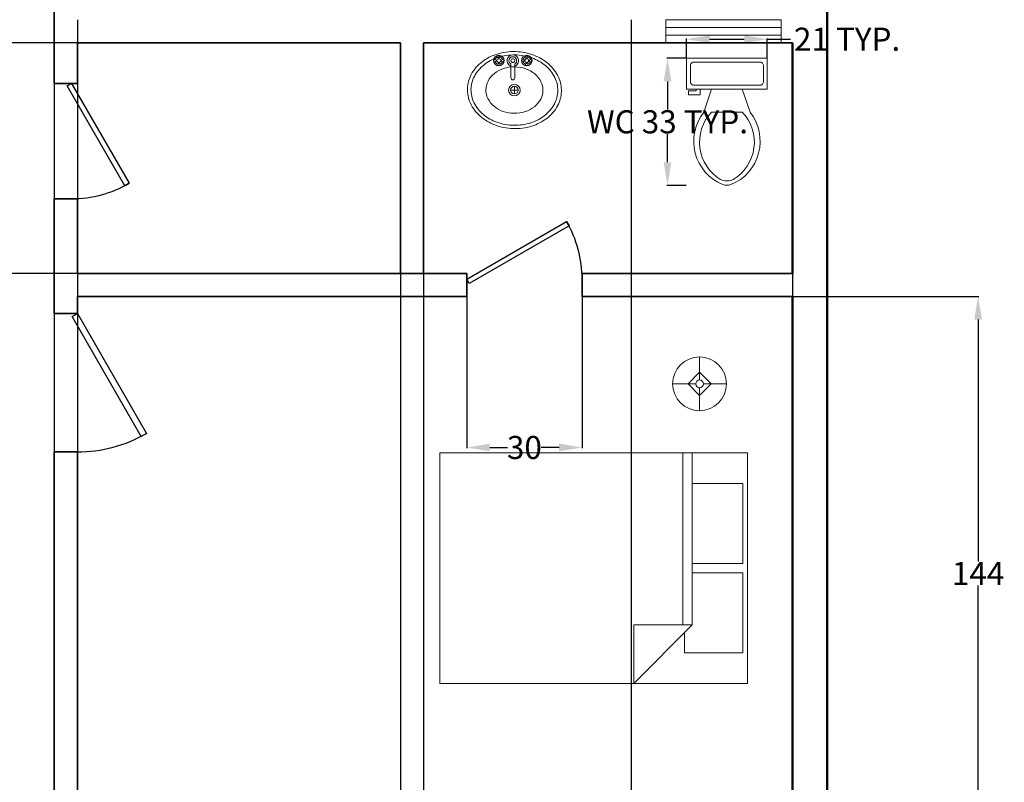
# Model space of a CAD drawing. Units: inches. Extents: x 823 to 1335, y 207 to 1074.
# Tile 5 of 6: x 1079 to 1335, y 577 to 776. Entities that reach past the tile are written whole.
import ezdxf

# ---------------------------------------------------------------- set-up
doc = ezdxf.new("R2010")
doc.units = ezdxf.units.IN
doc.header["$MEASUREMENT"] = 0
for name, color, linetype, lineweight in [('A-ANNO-DIMS', 2, 'Continuous', 18), ('doors', 51, 'Continuous', 25), ('furniture', 21, 'Continuous', 18), ('inner wall', 102, 'Continuous', 35), ('outer wall', 105, 'Continuous', 50), ('sanitary', 131, 'Continuous', 18), ('windows', 211, 'Continuous', 18)]:
    doc.layers.add(name, color=color, linetype=linetype, lineweight=lineweight)
doc.styles.get("Standard").update_dxf_attribs({"font": 'arial.ttf'})
doc.dimstyles.get("Standard").update_dxf_attribs({"dimtxt": 6, "dimasz": 6, "dimexe": 0.18, "dimexo": 0.0625, "dimgap": 0.09, "dimtad": 0, "dimtih": 1, "dimtoh": 1, "dimdec": 0, "dimzin": 0, "dimdsep": 46, "dimlunit": 3, "dimtxsty": 'Standard', "dimcen": 0.09, "dimadec": 0, "dimazin": 0, "dimtfac": 1, "dimtdec": 0, "dimtofl": 0, "dimtmove": 0, "dimatfit": 3, "dimfxl": 1, "dimtolj": 1, "dimtzin": 0, "dimarcsym": 0})

# ---------------------------------------------------------------- blocks, each defined once
blk = doc.blocks.new('*U4')
for p, q in [((-40, 0), (-40, 6)), ((0, 0), (0, 6))]:
    blk.add_line(p, q)
blk.add_lwpolyline([(0, 0), (-34.64, -20), (-35.52, -18.48), (-0.88, 1.52)], close=True)
blk.add_arc((0, 0), 40, 180, 210)
blk = doc.blocks.new('*U6')
for p, q in [((0, 0), (0, -6)), ((40, 0), (40, -6))]:
    blk.add_line(p, q)
blk.add_lwpolyline([(0, 0), (34.64, 20), (35.52, 18.48), (0.88, -1.52)], close=True)
blk.add_arc((0, 0), 40, 0, 30)
blk = doc.blocks.new('Bed - Queen')
for p, q in [((0, -80.00003), (0, 0)), ((0, 0), (59.99999, 0)), ((59.99999, 0), (59.99999, -80.00003)), ((7.99999, -1.2), (28.79998, -1.2)), ((7.99999, -14.4), (7.99999, -1.2)), ((28.79998, -1.2), (28.79998, -14.4)), ((31.19999, -1.2), (51.99999, -1.2)), ((31.19999, -14.4), (31.19999, -1.2)), ((51.99999, -1.2), (51.99999, -16.4)), ((0, -14.4), (44.8, -14.4)), ((59.99999, -29.6), (44.8, -14.4)), ((44.8, -14.4), (44.8, -29.6)), ((44.8, -16.8), (0, -16.8)), ((51.99999, -16.4), (46.79936, -16.4)), ((44.8, -29.6), (59.99999, -29.6)), ((59.99999, -80.00003), (0, -80.00003))]:
    blk.add_line(p, q)
blk = doc.blocks.new('Lamp - Table')
for p, q in [((0, 7), (0, 1)), ((0, 3), (-3, 0)), ((3, 0), (0, 3)), ((-1, 0), (-7, 0)), ((-3, 0), (0, -3)), ((0, -3), (3, 0)), ((1, 0), (7, 0)), ((0, -1), (0, -7))]:
    blk.add_line(p, q)
for radius in [7, 1]:
    blk.add_circle((0, 0), radius)
blk = doc.blocks.new('Sink - Oval top')
for p, q in [((-1, 0), (1, 0)), ((0, 1), (0, -1))]:
    blk.add_line(p, q)
for points in [[(-12.23, 0.39, 0.117634), (-11.46, -3.36, 0.104469), (-8.88, -6.8, 0.090016), (-5.08, -9.07, 0.08192), (-0.32, -10.02, 0.08192), (4.49, -9.38, 0.090016), (8.42, -7.36, 0.104469), (11.22, -4.09, 0.117634), (12.23, -0.39, 0.117634), (11.46, 3.36, 0.104469), (8.88, 6.8, 0.090016), (5.08, 9.07, 0.08192), (0.32, 10.02, 0.08192), (-4.49, 9.38, 0.090016), (-8.42, 7.36, 0.104469), (-11.22, 4.09, 0.117634)], [(-11.29, 0.16, 0.118622), (-10.52, -3.25, 0.104678), (-8.07, -6.36, 0.089562), (-4.54, -8.37, 0.081185), (-0.13, -9.15, 0.081185), (4.3, -8.49, 0.089562), (7.89, -6.58, 0.104678), (10.42, -3.55, 0.118622), (11.29, -0.16, 0.118622), (10.52, 3.25, 0.104678), (8.07, 6.36, 0.089562), (4.54, 8.37, 0.081185), (0.13, 9.15, 0.081185), (-4.3, 8.49, 0.089562), (-7.89, 6.58, 0.104678), (-10.42, 3.55, 0.118622)], [(-7.42, 0.08, 0.118283), (-6.91, -2.17, 0.104607), (-5.29, -4.21, 0.089718), (-2.97, -5.53, 0.081436), (-0.07, -6.04, 0.081436), (2.84, -5.59, 0.089718), (5.2, -4.33, 0.104607), (6.86, -2.32, 0.118283), (7.42, -0.08, 0.118283), (6.91, 2.17, 0.104607), (5.29, 4.21, 0.089718), (2.97, 5.53, 0.081436), (0.07, 6.04, 0.081436), (-2.84, 5.59, 0.089718), (-5.2, 4.33, 0.104607), (-6.86, 2.32, 0.118283)]]:
    blk.add_lwpolyline(points, format="xyb", close=True)
for radius in [1.5, 1]:
    blk.add_circle((0, 0), radius)
blk = doc.blocks.new('Faucet - Bathroom top')
for p, q in [((-4.107, 0.125), (-4.375, 0.125)), ((-3.75, 0.4788), (-3.75, 0.75)), ((-3.5, 0.482), (-3.5, 0.75)), ((-3.1461, 0.125), (-2.875, 0.125)), ((3.143, 0.125), (2.875, 0.125)), ((3.5, 0.4788), (3.5, 0.75)), ((3.75, 0.482), (3.75, 0.75)), ((4.1039, 0.125), (4.375, 0.125)), ((-4.1039, -0.125), (-4.375, -0.125)), ((-3.75, -0.4821), (-3.75, -0.75)), ((-3.5, -0.4789), (-3.5, -0.75)), ((-3.143, -0.125), (-2.875, -0.125)), ((-0.5, -0.8639), (-0.5, -4.5)), ((0.5, -4.5), (0.5, -0.8631)), ((3.1461, -0.125), (2.875, -0.125)), ((3.5, -0.4821), (3.5, -0.75)), ((3.75, -0.4789), (3.75, -0.75)), ((4.107, -0.125), (4.375, -0.125))]:
    blk.add_line(p, q)
for centre, radius in [((-3.625, 0), 1.375), ((-4.625, 0), 0.2795), ((-3.625, 0), 0.5), ((-3.625, 1), 0.2795), ((-2.625, 0), 0.2795), ((0, 0), 0.5), ((3.625, 0), 1.375), ((2.625, 0), 0.2795), ((3.625, 0), 0.5), ((3.625, 1), 0.2795), ((4.625, 0), 0.2795), ((-3.625, -1), 0.2795), ((3.625, -1), 0.2795)]:
    blk.add_circle(centre, radius)
for centre, radius, start, end in [((-3.625, 0), 1, 105.2407, 164.2093), ((-3.625, 0), 1, 16.44125, 74.07887), ((0, 0), 1.5, 289.6514, 250.3603), ((0, 0), 1, 300.3431, 239.7554), ((3.625, 0), 1, 106.12, 164.0884), ((3.625, 0), 1, 16.23422, 73.90469), ((-3.625, 0), 1, 196.2342, 253.9047), ((-3.625, 0), 1, 286.12, 344.0884), ((3.625, 0), 1, 196.4413, 254.0789), ((3.625, 0), 1, 285.2407, 344.2093), ((0, -4.5), 0.5, 180, 0)]:
    blk.add_arc(centre, radius, start, end)
blk = doc.blocks.new('Toilet - top')
for p, q in [((9.5, -6), (9.5, -2)), ((-10, -8.5), (-8, -8.5)), ((-10, -9.5), (-10, -8.5)), ((-7, -9.5), (-10, -9.5)), ((-8, -8.5), (-8, -8)), ((-7, -8), (-7, -9.5)), ((-4, -8), (-6, -14)), ((4, -8), (6, -14)), ((4, -14), (-4, -14))]:
    blk.add_line(p, q)
blk.add_lwpolyline([(10.5, -8), (10.5, 0), (-10.5, 0), (-10.5, -8)], close=True)
for points in [[(-9.5, -2), (-9.5, -6)], [(8.5, -1), (-8.5, -1)], [(-8.5, -7), (8.5, -7)]]:
    blk.add_lwpolyline(points)
for centre, radius, start, end in [((-8.62, -1.88), 0.884, 81.8699, 188.1301), ((8.62, -1.88), 0.884, 351.8699, 98.1301), ((-8.62, -6.12), 0.884, 171.8699, 278.1301), ((8.62, -6.12), 0.884, 261.8699, 8.1301), ((3.52, -21.58), 12.17, 141.4691, 247.9714), ((4.2, -21.82), 11.33, 136.3677, 238.9468), ((-3.52, -21.58), 12.17, 292.0284, 38.5307), ((-4.2, -21.82), 11.33, 301.053, 43.6321), ((0, -27.88), 4, 245.7318, 294.2682), ((0, -29), 4, 254.8605, 285.1395)]:
    blk.add_arc(centre, radius, start, end)
blk = doc.blocks.new('WIN-30IN')
for p, q in [((0, 6), (30, 6)), ((0, 0), (0, 6)), ((30, 6), (30, 0)), ((0, 4), (30, 4)), ((30, 2), (0, 2)), ((30, 0), (0, 0))]:
    blk.add_line(p, q)
blk = doc.blocks.new('*D44')
at = {"layer": 'A-ANNO-DIMS', "color": 0, "lineweight": -2, "transparency": 16777216}
for p, q in [((1252.63, 765.57), (1247.56, 765.57)), ((1247.74, 759.57), (1247.74, 752.24)), ((1247.74, 738.52), (1247.74, 745.85)), ((1252.63, 732.52), (1247.56, 732.52))]:
    blk.add_line(p, q, dxfattribs=at)
for points in [[(1246.74, 759.57), (1248.74, 759.57), (1247.74, 765.57)], [(1246.74, 738.52), (1248.74, 738.52), (1247.74, 732.52)]]:
    blk.add_solid(points, dxfattribs=at)
at = {"layer": 'Defpoints', "color": 0, "lineweight": -2, "transparency": 16777216}
for p in [(1247.74, 765.57), (1252.69, 765.57), (1252.69, 732.52)]:
    blk.add_point(p, dxfattribs=at)
at = {"layer": 'A-ANNO-DIMS', "color": 0, "transparency": 16777216, "insert": (1247.74, 749.05), "char_height": 6, "attachment_point": 5}
blk.add_mtext('\\A1;WC 33 TYP.', dxfattribs=at)
blk = doc.blocks.new('*D45')
at = {"layer": 'A-ANNO-DIMS', "color": 0, "lineweight": -2, "transparency": 16777216}
for p, q in [((1252.69, 765.63), (1252.69, 770.71)), ((1258.69, 770.53), (1267.69, 770.53)), ((1273.69, 765.63), (1273.69, 770.71)), ((1273.69, 770.53), (1279.69, 770.53))]:
    blk.add_line(p, q, dxfattribs=at)
for points in [[(1258.69, 771.53), (1258.69, 769.53), (1252.69, 770.53)], [(1267.69, 771.53), (1267.69, 769.53), (1273.69, 770.53)]]:
    blk.add_solid(points, dxfattribs=at)
at = {"layer": 'Defpoints', "color": 0, "lineweight": -2, "transparency": 16777216}
for p in [(1273.69, 770.53), (1252.69, 765.57), (1273.69, 765.57)]:
    blk.add_point(p, dxfattribs=at)
at = {"layer": 'A-ANNO-DIMS', "color": 0, "transparency": 16777216, "insert": (1294.44, 770.53), "char_height": 6, "attachment_point": 5}
blk.add_mtext('\\A1;21 TYP.', dxfattribs=at)
blk = doc.blocks.new('*D61')
at = {"layer": 'A-ANNO-DIMS', "color": 0, "lineweight": -2, "transparency": 16777216}
for p, q in [((1028.26, 847.54), (1028.26, 211.18)), ((1088.26, 847.54), (1088.26, 211.18)), ((1034.26, 211.36), (1053.87, 211.36)), ((1082.26, 211.36), (1062.66, 211.36))]:
    blk.add_line(p, q, dxfattribs=at)
for points in [[(1034.26, 212.36), (1034.26, 210.36), (1028.26, 211.36)], [(1082.26, 212.36), (1082.26, 210.36), (1088.26, 211.36)]]:
    blk.add_solid(points, dxfattribs=at)
at = {"layer": 'Defpoints', "color": 0, "lineweight": -2, "transparency": 16777216}
for p in [(1028.26, 847.61), (1088.26, 847.61), (1088.26, 211.36)]:
    blk.add_point(p, dxfattribs=at)
at = {"layer": 'A-ANNO-DIMS', "color": 0, "transparency": 16777216, "insert": (1058.26, 211.36), "char_height": 6, "attachment_point": 5}
blk.add_mtext('\\A1;60', dxfattribs=at)
blk = doc.blocks.new('*D62')
at = {"layer": 'A-ANNO-DIMS', "color": 0, "lineweight": -2, "transparency": 16777216}
for p, q in [((1094.26, 775.54), (1094.26, 211.18)), ((1238.26, 775.54), (1238.26, 211.18)), ((1100.26, 211.36), (1159.84, 211.36)), ((1232.26, 211.36), (1172.69, 211.36))]:
    blk.add_line(p, q, dxfattribs=at)
for points in [[(1100.26, 212.36), (1100.26, 210.36), (1094.26, 211.36)], [(1232.26, 212.36), (1232.26, 210.36), (1238.26, 211.36)]]:
    blk.add_solid(points, dxfattribs=at)
at = {"layer": 'Defpoints', "color": 0, "lineweight": -2, "transparency": 16777216}
for p in [(1094.26, 775.61), (1238.26, 775.61), (1238.26, 211.36)]:
    blk.add_point(p, dxfattribs=at)
at = {"layer": 'A-ANNO-DIMS', "color": 0, "transparency": 16777216, "insert": (1166.26, 211.36), "char_height": 6, "attachment_point": 5}
blk.add_mtext('\\A1;144', dxfattribs=at)
blk = doc.blocks.new('*D68')
at = {"layer": 'A-ANNO-DIMS', "color": 0, "lineweight": -2, "transparency": 16777216}
for p, q in [((1094.26, 709.54), (1094.26, 211.18)), ((1178.26, 709.54), (1178.26, 211.18)), ((1100.26, 211.36), (1131.88, 211.36)), ((1172.26, 211.36), (1140.64, 211.36))]:
    blk.add_line(p, q, dxfattribs=at)
for points in [[(1100.26, 212.36), (1100.26, 210.36), (1094.26, 211.36)], [(1172.26, 212.36), (1172.26, 210.36), (1178.26, 211.36)]]:
    blk.add_solid(points, dxfattribs=at)
at = {"layer": 'Defpoints', "color": 0, "lineweight": -2, "transparency": 16777216}
for p in [(1094.26, 709.61), (1178.26, 709.61), (1178.26, 211.36)]:
    blk.add_point(p, dxfattribs=at)
at = {"layer": 'A-ANNO-DIMS', "color": 0, "transparency": 16777216, "insert": (1136.26, 211.36), "char_height": 6, "attachment_point": 5}
blk.add_mtext('\\A1;84', dxfattribs=at)
blk = doc.blocks.new('*D69')
at = {"layer": 'A-ANNO-DIMS', "color": 0, "lineweight": -2, "transparency": 16777216}
for p, q in [((1184.26, 709.54), (1184.26, 211.18)), ((1280.26, 709.54), (1280.26, 211.18)), ((1190.26, 211.36), (1227.88, 211.36)), ((1274.26, 211.36), (1236.65, 211.36))]:
    blk.add_line(p, q, dxfattribs=at)
for points in [[(1190.26, 212.36), (1190.26, 210.36), (1184.26, 211.36)], [(1274.26, 212.36), (1274.26, 210.36), (1280.26, 211.36)]]:
    blk.add_solid(points, dxfattribs=at)
at = {"layer": 'Defpoints', "color": 0, "lineweight": -2, "transparency": 16777216}
for p in [(1184.26, 709.61), (1280.26, 709.61), (1280.26, 211.36)]:
    blk.add_point(p, dxfattribs=at)
at = {"layer": 'A-ANNO-DIMS', "color": 0, "transparency": 16777216, "insert": (1232.26, 211.36), "char_height": 6, "attachment_point": 5}
blk.add_mtext('\\A1;96', dxfattribs=at)
blk = doc.blocks.new('*D70')
at = {"layer": 'A-ANNO-DIMS', "color": 0, "lineweight": -2, "transparency": 16777216}
for p, q in [((1094.2, 769.61), (829.83, 769.61)), ((830.01, 763.61), (830.01, 742.76)), ((830.01, 715.61), (830.01, 736.45)), ((1094.2, 709.61), (829.83, 709.61))]:
    blk.add_line(p, q, dxfattribs=at)
for points in [[(829.01, 763.61), (831.01, 763.61), (830.01, 769.61)], [(829.01, 715.61), (831.01, 715.61), (830.01, 709.61)]]:
    blk.add_solid(points, dxfattribs=at)
at = {"layer": 'Defpoints', "color": 0, "lineweight": -2, "transparency": 16777216}
for p in [(1094.26, 769.61), (830.01, 709.61), (1094.26, 709.61)]:
    blk.add_point(p, dxfattribs=at)
at = {"layer": 'A-ANNO-DIMS', "color": 0, "transparency": 16777216, "insert": (830.01, 739.61), "char_height": 6, "attachment_point": 5}
blk.add_mtext('\\A1;60', dxfattribs=at)
blk = doc.blocks.new('*D72')
at = {"layer": 'A-ANNO-DIMS', "color": 0, "lineweight": -2, "transparency": 16777216}
for p, q in [((1280.32, 703.61), (1328.69, 703.61)), ((1328.51, 697.61), (1328.51, 634.71)), ((1328.51, 565.61), (1328.51, 628.5)), ((1280.32, 559.61), (1328.69, 559.61))]:
    blk.add_line(p, q, dxfattribs=at)
for points in [[(1327.51, 697.61), (1329.51, 697.61), (1328.51, 703.61)], [(1327.51, 565.61), (1329.51, 565.61), (1328.51, 559.61)]]:
    blk.add_solid(points, dxfattribs=at)
at = {"layer": 'Defpoints', "color": 0, "lineweight": -2, "transparency": 16777216}
for p in [(1280.26, 703.61), (1328.51, 703.61), (1280.26, 559.61)]:
    blk.add_point(p, dxfattribs=at)
at = {"layer": 'A-ANNO-DIMS', "color": 0, "transparency": 16777216, "insert": (1328.51, 631.61), "char_height": 6, "attachment_point": 5}
blk.add_mtext('\\A1;144', dxfattribs=at)
blk = doc.blocks.new('*D83')
at = {"layer": 'A-ANNO-DIMS', "color": 0, "lineweight": -2, "transparency": 16777216}
for p, q in [((1195.52, 703.54), (1195.52, 664.18)), ((1225.52, 703.54), (1225.52, 664.18)), ((1201.52, 664.36), (1206.15, 664.36)), ((1219.52, 664.36), (1214.9, 664.36))]:
    blk.add_line(p, q, dxfattribs=at)
for points in [[(1201.52, 665.36), (1201.52, 663.36), (1195.52, 664.36)], [(1219.52, 665.36), (1219.52, 663.36), (1225.52, 664.36)]]:
    blk.add_solid(points, dxfattribs=at)
at = {"layer": 'Defpoints', "color": 0, "lineweight": -2, "transparency": 16777216}
for p in [(1195.52, 703.61), (1225.52, 703.61), (1195.52, 664.36)]:
    blk.add_point(p, dxfattribs=at)
at = {"layer": 'A-ANNO-DIMS', "color": 0, "transparency": 16777216, "insert": (1210.52, 664.36), "char_height": 6, "attachment_point": 5}
blk.add_mtext('\\A1;30', dxfattribs=at)

msp = doc.modelspace()

# ---------------------------------------------------------------- linework, layer by layer
at = {"layer": 'inner wall'}
for p, q in [((1088.26, 779.51), (1088.26, 759.05)), ((1094.26, 769.61), (1178.26, 769.61)), ((1094.26, 769.61), (1094.26, 759.05)), ((1178.26, 769.61), (1178.26, 709.61)), ((1184.26, 769.61), (1184.26, 709.61)), ((1184.26, 769.61), (1280.26, 769.61)), ((1088.26, 729.05), (1088.26, 699.21)), ((1094.26, 729.05), (1094.26, 709.61)), ((1094.26, 709.61), (1195.52, 709.61)), ((1225.52, 709.61), (1280.26, 709.61)), ((1094.26, 703.61), (1195.52, 703.61)), ((1094.26, 703.61), (1094.26, 699.21)), ((1225.52, 703.61), (1280.26, 703.61)), ((1088.26, 663.21), (1088.26, 559.61)), ((1094.26, 663.21), (1094.26, 559.61))]:
    msp.add_line(p, q, dxfattribs=at)
for points in [[(1088.26, 759.05), (1094.26, 759.05)], [(1094.26, 729.05), (1088.26, 729.05)], [(1195.52, 703.61), (1195.52, 709.61)], [(1225.52, 709.61), (1225.52, 703.61)], [(1094.26, 699.21), (1088.26, 699.21)], [(1088.26, 663.21), (1094.26, 663.21)]]:
    msp.add_lwpolyline(points, dxfattribs=at)
at = {"layer": 'outer wall'}
for p, q in [((1280.26, 769.61), (1280.26, 709.61)), ((1280.26, 703.61), (1280.26, 559.61))]:
    msp.add_line(p, q, dxfattribs=at)
msp.add_lwpolyline([(869.26, 1030.61), (1289.26, 1030.61), (1289.26, 250.61), (869.26, 250.61)], close=True, dxfattribs=at)

# ---------------------------------------------------------------- block references
at = {"layer": 'doors'}
for name, p, xscale, yscale, zscale, rotation in [('*U6', (1092.76, 759.05), 0.75, 0.75, 0.75, 270), ('*U4', (1094.26, 699.21), 0.9, 0.9, 0.9, 90)]:
    msp.add_blockref(name, p, dxfattribs=dict(at, xscale=xscale, yscale=yscale, zscale=zscale, rotation=rotation))
at = {"layer": 'doors', "xscale": 0.75, "yscale": 0.75, "zscale": 0.75}
msp.add_blockref('*U6', (1195.52, 708.11), dxfattribs=at)
at = {"layer": 'furniture', "rotation": 270}
for name, p in [('Lamp - Table', (1256.07, 680.91)), ('Bed - Queen', (1268.56, 663))]:
    msp.add_blockref(name, p, dxfattribs=at)
at = {"layer": 'sanitary', "rotation": 180}
msp.add_blockref('Sink - Oval top', (1207.92, 757.3), dxfattribs=at)
at = {"layer": 'sanitary'}
for name, p in [('Faucet - Bathroom top', (1207.5, 764.97)), ('Toilet - top', (1263.19, 765.57))]:
    msp.add_blockref(name, p, dxfattribs=at)
at = {"layer": 'windows'}
msp.add_blockref('WIN-30IN', (1247.3, 769.61), dxfattribs=at)

# ---------------------------------------------------------------- dimensions: what is measured, and where the dimension line sits
at = {"layer": 'A-ANNO-DIMS'}
for base, p1, p2, picture, middle in [((1088.26, 211.36), (1028.26, 847.61), (1088.26, 847.61), '*D61', (1058.26, 211.36)), ((1238.26, 211.36), (1094.26, 775.61), (1238.26, 775.61), '*D62', (1166.26, 211.36)), ((1178.26, 211.36), (1094.26, 709.61), (1178.26, 709.61), '*D68', (1136.26, 211.36)), ((1280.26, 211.36), (1184.26, 709.61), (1280.26, 709.61), '*D69', (1232.26, 211.36))]:
    dim = msp.add_linear_dim(base=base, p1=p1, p2=p2, dimstyle='Standard', override={"dimdec": 0, "dimlfac": 1, "dimrnd": 0, "dimzin": 0, "dimdsep": 46, "dimlunit": 2}, dxfattribs=at)
    dim.commit()
    dim.dimension.update_dxf_attribs({"geometry": picture, "text_midpoint": middle})
dim = msp.add_linear_dim(base=(1273.69, 770.53), p1=(1252.69, 765.57), p2=(1273.69, 765.57), text='<> TYP.', dimstyle='Standard', override={"dimdec": 0, "dimlfac": 1, "dimrnd": 0, "dimzin": 0, "dimdsep": 46, "dimlunit": 2}, dxfattribs=at)
dim.commit()
dim.dimension.update_dxf_attribs({"geometry": '*D45', "text_midpoint": (1294.44, 770.53)})
for base, p1, p2, angle, picture, middle in [((830.01, 709.61), (1094.26, 769.61), (1094.26, 709.61), 90, '*D70', (830.01, 739.61)), ((1195.52, 664.36), (1225.52, 703.61), (1195.52, 703.61), 180, '*D83', (1210.52, 664.36)), ((1328.51, 703.61), (1280.26, 559.61), (1280.26, 703.61), 90, '*D72', (1328.51, 631.61))]:
    dim = msp.add_linear_dim(base=base, p1=p1, p2=p2, angle=angle, dimstyle='Standard', override={"dimdec": 0, "dimlfac": 1, "dimrnd": 0, "dimzin": 0, "dimdsep": 46, "dimlunit": 2}, dxfattribs=at)
    dim.commit()
    dim.dimension.update_dxf_attribs({"geometry": picture, "text_midpoint": middle})
dim = msp.add_linear_dim(base=(1247.74, 765.57), p1=(1252.69, 732.52), p2=(1252.69, 765.57), angle=90, text='WC <> TYP.', dimstyle='Standard', override={"dimdec": 0, "dimlfac": 1, "dimrnd": 0, "dimzin": 0, "dimdsep": 46, "dimlunit": 2}, dxfattribs=at)
dim.commit()
dim.dimension.update_dxf_attribs({"geometry": '*D44', "text_midpoint": (1247.74, 749.05)})

doc.saveas('drawing.dxf')
